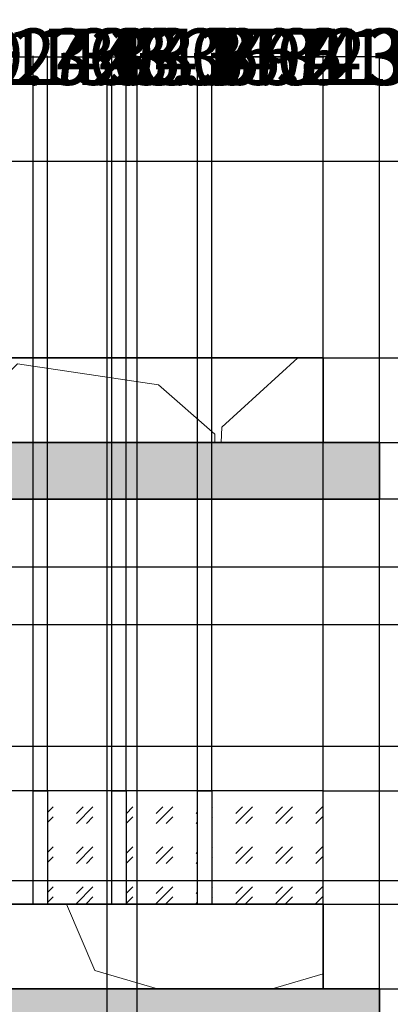
# Model space of a CAD drawing. Units: inches. Extents: x -73 to 458, y -161 to 332.
# Tile 5 of 6: x 259 to 338, y 123 to 332. Entities that reach past the tile are written whole.
import ezdxf

# ---------------------------------------------------------------- set-up
doc = ezdxf.new("R2010")
doc.units = ezdxf.units.IN
doc.header["$MEASUREMENT"] = 0
for name, color, linetype, lineweight in [('A-ANNO-DIMS', 2, 'Continuous', 18), ('A-ELEV', 7, 'Continuous', 35), ('A-ELEV-PATT', 8, 'Continuous', 13), ('A-GLAZ', 3, 'Continuous', 25), ('A-GLAZ-PATT', 8, 'Continuous', 13)]:
    doc.layers.add(name, color=color, linetype=linetype, lineweight=lineweight)
doc.styles.get("Standard").update_dxf_attribs({"font": 'arial.ttf'})
doc.dimstyles.get("Standard").update_dxf_attribs({"dimtxt": 12, "dimasz": 0.18, "dimexe": 0.18, "dimexo": 0.0625, "dimgap": 0.09, "dimtad": 0, "dimtih": 1, "dimtoh": 1, "dimdec": 0, "dimzin": 0, "dimdsep": 46, "dimlunit": 3, "dimtxsty": 'Standard', "dimcen": 0.09, "dimadec": 0, "dimazin": 0, "dimtfac": 1, "dimtdec": 0, "dimtofl": 0, "dimtmove": 0, "dimatfit": 3, "dimfxl": 1, "dimtolj": 1, "dimtzin": 0, "dimarcsym": 0})

# ---------------------------------------------------------------- blocks, each defined once
blk = doc.blocks.new('*D8')
at = {"layer": 'A-ANNO-DIMS', "color": 0, "lineweight": -2, "transparency": 16777216}
for p, q in [((204, 24.13), (204, 324.4)), ((204.18, 324.22), (257.28, 324.22)), ((335.82, 324.22), (282.72, 324.22)), ((336, 126.13), (336, 324.4))]:
    blk.add_line(p, q, dxfattribs=at)
at = {"layer": 'A-ANNO-DIMS', "color": 0, "transparency": 16777216}
for points in [[(204.18, 324.25), (204.18, 324.19), (204, 324.22)], [(335.82, 324.25), (335.82, 324.19), (336, 324.22)]]:
    blk.add_solid(points, dxfattribs=at)
at = {"layer": 'Defpoints', "color": 0, "transparency": 16777216}
for p in [(336, 324.22), (336, 126.07), (204, 24.07)]:
    blk.add_point(p, dxfattribs=at)
at = {"layer": 'A-ANNO-DIMS', "color": 0, "transparency": 16777216, "insert": (270, 324.22), "char_height": 12, "attachment_point": 5}
blk.add_mtext('\\A1;132', dxfattribs=at)
blk = doc.blocks.new('*D21')
at = {"layer": 'A-ANNO-DIMS', "color": 0, "lineweight": -2, "transparency": 16777216}
for p, q in [((336.06, 126.07), (408.51, 126.07)), ((408.33, 126.07), (408.33, 126.25)), ((408.33, 126.25), (408.51, 126.25)), ((408.33, 114.25), (408.33, 125.89)), ((336.06, 114.07), (408.51, 114.07))]:
    blk.add_line(p, q, dxfattribs=at)
at = {"layer": 'A-ANNO-DIMS', "color": 0, "transparency": 16777216}
for points in [[(408.3, 125.89), (408.36, 125.89), (408.33, 126.07)], [(408.3, 114.25), (408.36, 114.25), (408.33, 114.07)]]:
    blk.add_solid(points, dxfattribs=at)
at = {"layer": 'Defpoints', "color": 0, "transparency": 16777216}
for p in [(336, 126.07), (408.33, 126.07), (336, 114.07)]:
    blk.add_point(p, dxfattribs=at)
at = {"layer": 'A-ANNO-DIMS', "color": 0, "transparency": 16777216, "insert": (416.56, 126.25), "char_height": 12, "attachment_point": 5}
blk.add_mtext('\\A1;12', dxfattribs=at)
blk = doc.blocks.new('*D22')
at = {"layer": 'A-ANNO-DIMS', "color": 0, "lineweight": -2, "transparency": 16777216}
for p, q in [((336.06, 230.21), (408.51, 230.21)), ((408.33, 230.03), (408.33, 184.35)), ((408.33, 126.25), (408.33, 171.92)), ((336.06, 126.07), (408.51, 126.07))]:
    blk.add_line(p, q, dxfattribs=at)
at = {"layer": 'A-ANNO-DIMS', "color": 0, "transparency": 16777216}
for points in [[(408.3, 230.03), (408.36, 230.03), (408.33, 230.21)], [(408.3, 126.25), (408.36, 126.25), (408.33, 126.07)]]:
    blk.add_solid(points, dxfattribs=at)
at = {"layer": 'Defpoints', "color": 0, "transparency": 16777216}
for p in [(336, 230.21), (408.33, 230.21), (336, 126.07)]:
    blk.add_point(p, dxfattribs=at)
at = {"layer": 'A-ANNO-DIMS', "color": 0, "transparency": 16777216, "insert": (408.33, 178.14), "char_height": 12, "attachment_point": 5}
blk.add_mtext('\\A1;104.14', dxfattribs=at)
blk = doc.blocks.new('*D23')
at = {"layer": 'A-ANNO-DIMS', "color": 0, "lineweight": -2, "transparency": 16777216}
for p, q in [((336.06, 242.21), (408.51, 242.21)), ((408.33, 242.21), (408.33, 242.39)), ((408.33, 242.39), (408.51, 242.39)), ((408.33, 230.39), (408.33, 242.03)), ((336.06, 230.21), (408.51, 230.21))]:
    blk.add_line(p, q, dxfattribs=at)
at = {"layer": 'A-ANNO-DIMS', "color": 0, "transparency": 16777216}
for points in [[(408.3, 242.03), (408.36, 242.03), (408.33, 242.21)], [(408.3, 230.39), (408.36, 230.39), (408.33, 230.21)]]:
    blk.add_solid(points, dxfattribs=at)
at = {"layer": 'Defpoints', "color": 0, "transparency": 16777216}
for p in [(336, 242.21), (408.33, 242.21), (336, 230.21)]:
    blk.add_point(p, dxfattribs=at)
at = {"layer": 'A-ANNO-DIMS', "color": 0, "transparency": 16777216, "insert": (416.56, 242.39), "char_height": 12, "attachment_point": 5}
blk.add_mtext('\\A1;12', dxfattribs=at)
blk = doc.blocks.new('*D24')
at = {"layer": 'A-ANNO-DIMS', "color": 0, "lineweight": -2, "transparency": 16777216}
for p, q in [((324.06, 260.21), (408.51, 260.21)), ((408.33, 260.03), (408.33, 257.42)), ((408.33, 242.39), (408.33, 244.99)), ((324.06, 242.21), (408.51, 242.21))]:
    blk.add_line(p, q, dxfattribs=at)
at = {"layer": 'A-ANNO-DIMS', "color": 0, "transparency": 16777216}
for points in [[(408.3, 260.03), (408.36, 260.03), (408.33, 260.21)], [(408.3, 242.39), (408.36, 242.39), (408.33, 242.21)]]:
    blk.add_solid(points, dxfattribs=at)
at = {"layer": 'Defpoints', "color": 0, "transparency": 16777216}
for p in [(324, 260.21), (408.33, 260.21), (324, 242.21)]:
    blk.add_point(p, dxfattribs=at)
at = {"layer": 'A-ANNO-DIMS', "color": 0, "transparency": 16777216, "insert": (408.33, 251.21), "char_height": 12, "attachment_point": 5}
blk.add_mtext('\\A1;18', dxfattribs=at)
blk = doc.blocks.new('*D25')
at = {"layer": 'A-ANNO-DIMS', "color": 0, "lineweight": -2, "transparency": 16777216}
for p, q in [((168.06, 302.02), (408.51, 302.02)), ((408.33, 301.84), (408.33, 287.33)), ((408.33, 260.39), (408.33, 274.9)), ((168.06, 260.21), (408.51, 260.21))]:
    blk.add_line(p, q, dxfattribs=at)
at = {"layer": 'A-ANNO-DIMS', "color": 0, "transparency": 16777216}
for points in [[(408.3, 301.84), (408.36, 301.84), (408.33, 302.02)], [(408.3, 260.39), (408.36, 260.39), (408.33, 260.21)]]:
    blk.add_solid(points, dxfattribs=at)
at = {"layer": 'Defpoints', "color": 0, "transparency": 16777216}
for p in [(168, 302.02), (408.33, 302.02), (168, 260.21)]:
    blk.add_point(p, dxfattribs=at)
at = {"layer": 'A-ANNO-DIMS', "color": 0, "transparency": 16777216, "insert": (408.33, 281.11), "char_height": 12, "attachment_point": 5}
blk.add_mtext('\\A1;41.814', dxfattribs=at)
blk = doc.blocks.new('*D42')
at = {"layer": 'A-ANNO-DIMS', "color": 0, "lineweight": -2, "transparency": 16777216}
for p, q in [((144.06, 149.14), (408.51, 149.14)), ((408.33, 148.96), (408.33, 140.32)), ((408.33, 119.24), (408.33, 127.88)), ((144.06, 119.06), (408.51, 119.06))]:
    blk.add_line(p, q, dxfattribs=at)
at = {"layer": 'A-ANNO-DIMS', "color": 0, "transparency": 16777216}
for points in [[(408.3, 148.96), (408.36, 148.96), (408.33, 149.14)], [(408.3, 119.24), (408.36, 119.24), (408.33, 119.06)]]:
    blk.add_solid(points, dxfattribs=at)
at = {"layer": 'Defpoints', "color": 0, "transparency": 16777216}
for p in [(144, 149.14), (408.33, 149.14), (144, 119.06)]:
    blk.add_point(p, dxfattribs=at)
at = {"layer": 'A-ANNO-DIMS', "color": 0, "transparency": 16777216, "insert": (408.33, 134.1), "char_height": 12, "attachment_point": 5}
blk.add_mtext('\\A1;30.08', dxfattribs=at)
blk = doc.blocks.new('*D43')
at = {"layer": 'A-ANNO-DIMS', "color": 0, "lineweight": -2, "transparency": 16777216}
for p, q in [((144.06, 177.7), (408.51, 177.7)), ((408.33, 177.52), (408.33, 169.64)), ((408.33, 149.32), (408.33, 157.2)), ((144.06, 149.14), (408.51, 149.14))]:
    blk.add_line(p, q, dxfattribs=at)
at = {"layer": 'A-ANNO-DIMS', "color": 0, "transparency": 16777216}
for points in [[(408.3, 177.52), (408.36, 177.52), (408.33, 177.7)], [(408.3, 149.32), (408.36, 149.32), (408.33, 149.14)]]:
    blk.add_solid(points, dxfattribs=at)
at = {"layer": 'Defpoints', "color": 0, "transparency": 16777216}
for p in [(144, 177.7), (408.33, 177.7), (144, 149.14)]:
    blk.add_point(p, dxfattribs=at)
at = {"layer": 'A-ANNO-DIMS', "color": 0, "transparency": 16777216, "insert": (408.33, 163.42), "char_height": 12, "attachment_point": 5}
blk.add_mtext('\\A1;28.57', dxfattribs=at)
blk = doc.blocks.new('*D44')
at = {"layer": 'A-ANNO-DIMS', "color": 0, "lineweight": -2, "transparency": 16777216}
for p, q in [((144.06, 203.54), (408.51, 203.54)), ((408.33, 203.36), (408.33, 196.84)), ((408.33, 177.88), (408.33, 184.4)), ((144.06, 177.7), (408.51, 177.7))]:
    blk.add_line(p, q, dxfattribs=at)
at = {"layer": 'A-ANNO-DIMS', "color": 0, "transparency": 16777216}
for points in [[(408.3, 203.36), (408.36, 203.36), (408.33, 203.54)], [(408.3, 177.88), (408.36, 177.88), (408.33, 177.7)]]:
    blk.add_solid(points, dxfattribs=at)
at = {"layer": 'Defpoints', "color": 0, "transparency": 16777216}
for p in [(144, 203.54), (408.33, 203.54), (144, 177.7)]:
    blk.add_point(p, dxfattribs=at)
at = {"layer": 'A-ANNO-DIMS', "color": 0, "transparency": 16777216, "insert": (408.33, 190.62), "char_height": 12, "attachment_point": 5}
blk.add_mtext('\\A1;25.83', dxfattribs=at)
blk = doc.blocks.new('*D45')
at = {"layer": 'A-ANNO-DIMS', "color": 0, "lineweight": -2, "transparency": 16777216}
for p, q in [((144.06, 215.8), (408.51, 215.8)), ((408.33, 215.8), (408.33, 215.98)), ((408.33, 215.98), (408.51, 215.98)), ((408.33, 203.72), (408.33, 215.62)), ((144.06, 203.54), (408.51, 203.54))]:
    blk.add_line(p, q, dxfattribs=at)
at = {"layer": 'A-ANNO-DIMS', "color": 0, "transparency": 16777216}
for points in [[(408.3, 215.62), (408.36, 215.62), (408.33, 215.8)], [(408.3, 203.72), (408.36, 203.72), (408.33, 203.54)]]:
    blk.add_solid(points, dxfattribs=at)
at = {"layer": 'Defpoints', "color": 0, "transparency": 16777216}
for p in [(144, 215.8), (408.33, 215.8), (144, 203.54)]:
    blk.add_point(p, dxfattribs=at)
at = {"layer": 'A-ANNO-DIMS', "color": 0, "transparency": 16777216, "insert": (432.98, 215.98), "char_height": 12, "attachment_point": 5}
blk.add_mtext('\\A1;12.265', dxfattribs=at)
blk = doc.blocks.new('*D46')
at = {"layer": 'A-ANNO-DIMS', "color": 0, "lineweight": -2, "transparency": 16777216}
for p, q in [((156.06, 230.21), (408.51, 230.21)), ((408.33, 230.03), (408.33, 229.22)), ((144.06, 215.8), (408.51, 215.8)), ((408.33, 215.98), (408.33, 216.79))]:
    blk.add_line(p, q, dxfattribs=at)
at = {"layer": 'A-ANNO-DIMS', "color": 0, "transparency": 16777216}
for points in [[(408.3, 230.03), (408.36, 230.03), (408.33, 230.21)], [(408.3, 215.98), (408.36, 215.98), (408.33, 215.8)]]:
    blk.add_solid(points, dxfattribs=at)
at = {"layer": 'Defpoints', "color": 0, "transparency": 16777216}
for p in [(156, 230.21), (408.33, 230.21), (144, 215.8)]:
    blk.add_point(p, dxfattribs=at)
at = {"layer": 'A-ANNO-DIMS', "color": 0, "transparency": 16777216, "insert": (408.33, 223), "char_height": 12, "attachment_point": 5}
blk.add_mtext('\\A1;14.406', dxfattribs=at)
blk = doc.blocks.new('*D54')
at = {"layer": 'A-ANNO-DIMS', "color": 0, "lineweight": -2, "transparency": 16777216}
for p, q in [((249, 168.25), (249, 324.4)), ((249.18, 324.22), (262.15, 324.22)), ((262.33, 168.25), (262.33, 324.4)), ((262.33, 324.22), (262.51, 324.22))]:
    blk.add_line(p, q, dxfattribs=at)
at = {"layer": 'A-ANNO-DIMS', "color": 0, "transparency": 16777216}
for points in [[(249.18, 324.25), (249.18, 324.19), (249, 324.22)], [(262.15, 324.25), (262.15, 324.19), (262.33, 324.22)]]:
    blk.add_solid(points, dxfattribs=at)
at = {"layer": 'Defpoints', "color": 0, "transparency": 16777216}
for p in [(262.33, 324.22), (249, 168.19), (262.33, 168.19)]:
    blk.add_point(p, dxfattribs=at)
at = {"layer": 'A-ANNO-DIMS', "color": 0, "transparency": 16777216, "insert": (282.28, 324.22), "char_height": 12, "attachment_point": 5}
blk.add_mtext('\\A1;13.33', dxfattribs=at)
blk = doc.blocks.new('*D55')
at = {"layer": 'A-ANNO-DIMS', "color": 0, "lineweight": -2, "transparency": 16777216}
for p, q in [((262.33, 168.25), (262.33, 324.4)), ((262.51, 324.22), (265.19, 324.22)), ((265.37, 168.25), (265.37, 324.4)), ((265.37, 324.22), (265.55, 324.22))]:
    blk.add_line(p, q, dxfattribs=at)
at = {"layer": 'A-ANNO-DIMS', "color": 0, "transparency": 16777216}
for points in [[(262.51, 324.25), (262.51, 324.19), (262.33, 324.22)], [(265.19, 324.25), (265.19, 324.19), (265.37, 324.22)]]:
    blk.add_solid(points, dxfattribs=at)
at = {"layer": 'Defpoints', "color": 0, "transparency": 16777216}
for p in [(265.37, 324.22), (262.33, 168.19), (265.37, 168.19)]:
    blk.add_point(p, dxfattribs=at)
at = {"layer": 'A-ANNO-DIMS', "color": 0, "transparency": 16777216, "insert": (285.88, 324.22), "char_height": 12, "attachment_point": 5}
blk.add_mtext('\\A1;3.043', dxfattribs=at)
blk = doc.blocks.new('*D56')
at = {"layer": 'A-ANNO-DIMS', "color": 0, "lineweight": -2, "transparency": 16777216}
for p, q in [((265.37, 168.25), (265.37, 324.4)), ((265.55, 324.22), (278.88, 324.22)), ((279.06, 168.25), (279.06, 324.4)), ((279.06, 324.22), (279.24, 324.22))]:
    blk.add_line(p, q, dxfattribs=at)
at = {"layer": 'A-ANNO-DIMS', "color": 0, "transparency": 16777216}
for points in [[(265.55, 324.25), (265.55, 324.19), (265.37, 324.22)], [(278.88, 324.25), (278.88, 324.19), (279.06, 324.22)]]:
    blk.add_solid(points, dxfattribs=at)
at = {"layer": 'Defpoints', "color": 0, "transparency": 16777216}
for p in [(279.06, 324.22), (265.37, 168.19), (279.06, 168.19)]:
    blk.add_point(p, dxfattribs=at)
at = {"layer": 'A-ANNO-DIMS', "color": 0, "transparency": 16777216, "insert": (303.65, 324.22), "char_height": 12, "attachment_point": 5}
blk.add_mtext('\\A1;13.694', dxfattribs=at)
blk = doc.blocks.new('*D57')
at = {"layer": 'A-ANNO-DIMS', "color": 0, "lineweight": -2, "transparency": 16777216}
for p, q in [((279.06, 168.25), (279.06, 324.4)), ((279.24, 324.22), (281.93, 324.22)), ((282.11, 168.25), (282.11, 324.4)), ((282.11, 324.22), (282.29, 324.22))]:
    blk.add_line(p, q, dxfattribs=at)
at = {"layer": 'A-ANNO-DIMS', "color": 0, "transparency": 16777216}
for points in [[(279.24, 324.25), (279.24, 324.19), (279.06, 324.22)], [(281.93, 324.25), (281.93, 324.19), (282.11, 324.22)]]:
    blk.add_solid(points, dxfattribs=at)
at = {"layer": 'Defpoints', "color": 0, "transparency": 16777216}
for p in [(282.11, 324.22), (279.06, 168.19), (282.11, 168.19)]:
    blk.add_point(p, dxfattribs=at)
at = {"layer": 'A-ANNO-DIMS', "color": 0, "transparency": 16777216, "insert": (302.62, 324.22), "char_height": 12, "attachment_point": 5}
blk.add_mtext('\\A1;3.043', dxfattribs=at)
blk = doc.blocks.new('*D58')
at = {"layer": 'A-ANNO-DIMS', "color": 0, "lineweight": -2, "transparency": 16777216}
for p, q in [((282.11, 168.25), (282.11, 324.4)), ((282.29, 324.22), (297.14, 324.22)), ((297.32, 168.25), (297.32, 324.4)), ((297.32, 324.22), (297.5, 324.22))]:
    blk.add_line(p, q, dxfattribs=at)
at = {"layer": 'A-ANNO-DIMS', "color": 0, "transparency": 16777216}
for points in [[(282.29, 324.25), (282.29, 324.19), (282.11, 324.22)], [(297.14, 324.25), (297.14, 324.19), (297.32, 324.22)]]:
    blk.add_solid(points, dxfattribs=at)
at = {"layer": 'Defpoints', "color": 0, "transparency": 16777216}
for p in [(297.32, 324.22), (282.11, 168.19), (297.32, 168.19)]:
    blk.add_point(p, dxfattribs=at)
at = {"layer": 'A-ANNO-DIMS', "color": 0, "transparency": 16777216, "insert": (321.93, 324.22), "char_height": 12, "attachment_point": 5}
blk.add_mtext('\\A1;15.216', dxfattribs=at)
blk = doc.blocks.new('*D59')
at = {"layer": 'A-ANNO-DIMS', "color": 0, "lineweight": -2, "transparency": 16777216}
for p, q in [((297.32, 168.25), (297.32, 324.4)), ((297.5, 324.22), (300.19, 324.22)), ((300.37, 168.25), (300.37, 324.4)), ((300.37, 324.22), (300.55, 324.22))]:
    blk.add_line(p, q, dxfattribs=at)
at = {"layer": 'A-ANNO-DIMS', "color": 0, "transparency": 16777216}
for points in [[(297.5, 324.25), (297.5, 324.19), (297.32, 324.22)], [(300.19, 324.25), (300.19, 324.19), (300.37, 324.22)]]:
    blk.add_solid(points, dxfattribs=at)
at = {"layer": 'Defpoints', "color": 0, "transparency": 16777216}
for p in [(300.37, 324.22), (297.32, 168.19), (300.37, 168.19)]:
    blk.add_point(p, dxfattribs=at)
at = {"layer": 'A-ANNO-DIMS', "color": 0, "transparency": 16777216, "insert": (320.88, 324.22), "char_height": 12, "attachment_point": 5}
blk.add_mtext('\\A1;3.043', dxfattribs=at)
blk = doc.blocks.new('*D60')
at = {"layer": 'A-ANNO-DIMS', "color": 0, "lineweight": -2, "transparency": 16777216}
for p, q in [((300.37, 168.25), (300.37, 324.4)), ((300.55, 324.22), (323.82, 324.22)), ((324, 168.25), (324, 324.4)), ((324, 324.22), (324.18, 324.22))]:
    blk.add_line(p, q, dxfattribs=at)
at = {"layer": 'A-ANNO-DIMS', "color": 0, "transparency": 16777216}
for points in [[(300.55, 324.25), (300.55, 324.19), (300.37, 324.22)], [(323.82, 324.25), (323.82, 324.19), (324, 324.22)]]:
    blk.add_solid(points, dxfattribs=at)
at = {"layer": 'Defpoints', "color": 0, "transparency": 16777216}
for p in [(324, 324.22), (300.37, 168.19), (324, 168.19)]:
    blk.add_point(p, dxfattribs=at)
at = {"layer": 'A-ANNO-DIMS', "color": 0, "transparency": 16777216, "insert": (344.62, 324.22), "char_height": 12, "attachment_point": 5}
blk.add_mtext('\\A1;23.63', dxfattribs=at)
blk = doc.blocks.new('*D69')
at = {"layer": 'A-ANNO-DIMS', "color": 0, "lineweight": -2, "transparency": 16777216}
for p, q in [((324.06, 168.19), (408.51, 168.19)), ((408.33, 168.01), (408.33, 162.35)), ((408.33, 144.25), (408.33, 149.91)), ((324.06, 144.07), (408.51, 144.07))]:
    blk.add_line(p, q, dxfattribs=at)
at = {"layer": 'A-ANNO-DIMS', "color": 0, "transparency": 16777216}
for points in [[(408.3, 168.01), (408.36, 168.01), (408.33, 168.19)], [(408.3, 144.25), (408.36, 144.25), (408.33, 144.07)]]:
    blk.add_solid(points, dxfattribs=at)
at = {"layer": 'Defpoints', "color": 0, "transparency": 16777216}
for p in [(324, 168.19), (408.33, 168.19), (324, 144.07)]:
    blk.add_point(p, dxfattribs=at)
at = {"layer": 'A-ANNO-DIMS', "color": 0, "transparency": 16777216, "insert": (408.33, 156.13), "char_height": 12, "attachment_point": 5}
blk.add_mtext('\\A1;24.125', dxfattribs=at)
blk = doc.blocks.new('*D72')
at = {"layer": 'A-ANNO-DIMS', "color": 0, "lineweight": -2, "transparency": 16777216}
for p, q in [((202.35, -5.87), (202.35, 324.4)), ((202.53, 324.22), (241.93, 324.22)), ((242.11, -5.87), (242.11, 324.4)), ((242.11, 324.22), (242.29, 324.22))]:
    blk.add_line(p, q, dxfattribs=at)
at = {"layer": 'A-ANNO-DIMS', "color": 0, "transparency": 16777216}
for points in [[(202.53, 324.25), (202.53, 324.19), (202.35, 324.22)], [(241.93, 324.25), (241.93, 324.19), (242.11, 324.22)]]:
    blk.add_solid(points, dxfattribs=at)
at = {"layer": 'Defpoints', "color": 0, "transparency": 16777216}
for p in [(242.11, 324.22), (202.35, -5.93), (242.11, -5.93)]:
    blk.add_point(p, dxfattribs=at)
at = {"layer": 'A-ANNO-DIMS', "color": 0, "transparency": 16777216, "insert": (262.62, 324.22), "char_height": 12, "attachment_point": 5}
blk.add_mtext('\\A1;39.76', dxfattribs=at)
blk = doc.blocks.new('*D73')
at = {"layer": 'A-ANNO-DIMS', "color": 0, "lineweight": -2, "transparency": 16777216}
for p, q in [((242.11, -5.87), (242.11, 324.4)), ((242.29, 324.22), (244.17, 324.22)), ((244.35, -5.87), (244.35, 324.4)), ((244.35, 324.22), (244.53, 324.22))]:
    blk.add_line(p, q, dxfattribs=at)
at = {"layer": 'A-ANNO-DIMS', "color": 0, "transparency": 16777216}
for points in [[(242.29, 324.25), (242.29, 324.19), (242.11, 324.22)], [(244.17, 324.25), (244.17, 324.19), (244.35, 324.22)]]:
    blk.add_solid(points, dxfattribs=at)
at = {"layer": 'Defpoints', "color": 0, "transparency": 16777216}
for p in [(244.35, 324.22), (242.11, -5.93), (244.35, -5.93)]:
    blk.add_point(p, dxfattribs=at)
at = {"layer": 'A-ANNO-DIMS', "color": 0, "transparency": 16777216, "insert": (264.95, 324.22), "char_height": 12, "attachment_point": 5}
blk.add_mtext('\\A1;2.244', dxfattribs=at)
blk = doc.blocks.new('*D74')
at = {"layer": 'A-ANNO-DIMS', "color": 0, "lineweight": -2, "transparency": 16777216}
for p, q in [((244.35, -5.87), (244.35, 324.4)), ((244.53, 324.22), (277.93, 324.22)), ((278.11, -5.87), (278.11, 324.4)), ((278.11, 324.22), (278.29, 324.22))]:
    blk.add_line(p, q, dxfattribs=at)
at = {"layer": 'A-ANNO-DIMS', "color": 0, "transparency": 16777216}
for points in [[(244.53, 324.25), (244.53, 324.19), (244.35, 324.22)], [(277.93, 324.25), (277.93, 324.19), (278.11, 324.22)]]:
    blk.add_solid(points, dxfattribs=at)
at = {"layer": 'Defpoints', "color": 0, "transparency": 16777216}
for p in [(278.11, 324.22), (244.35, -5.93), (278.11, -5.93)]:
    blk.add_point(p, dxfattribs=at)
at = {"layer": 'A-ANNO-DIMS', "color": 0, "transparency": 16777216, "insert": (303.28, 324.22), "char_height": 12, "attachment_point": 5}
blk.add_mtext('\\A1;33.756', dxfattribs=at)
blk = doc.blocks.new('*D75')
at = {"layer": 'A-ANNO-DIMS', "color": 0, "lineweight": -2, "transparency": 16777216}
for p, q in [((278.11, -5.87), (278.11, 324.4)), ((278.29, 324.22), (284.3, 324.22)), ((284.48, -5.87), (284.48, 324.4)), ((284.48, 324.22), (284.66, 324.22))]:
    blk.add_line(p, q, dxfattribs=at)
at = {"layer": 'A-ANNO-DIMS', "color": 0, "transparency": 16777216}
for points in [[(278.29, 324.25), (278.29, 324.19), (278.11, 324.22)], [(284.3, 324.25), (284.3, 324.19), (284.48, 324.22)]]:
    blk.add_solid(points, dxfattribs=at)
at = {"layer": 'Defpoints', "color": 0, "transparency": 16777216}
for p in [(284.48, 324.22), (278.11, -5.93), (284.48, -5.93)]:
    blk.add_point(p, dxfattribs=at)
at = {"layer": 'A-ANNO-DIMS', "color": 0, "transparency": 16777216, "insert": (305.03, 324.22), "char_height": 12, "attachment_point": 5}
blk.add_mtext('\\A1;6.377', dxfattribs=at)

msp = doc.modelspace()

# ---------------------------------------------------------------- hatches: boundary and pattern name
at = {"layer": 'A-ELEV-PATT'}
h = msp.add_hatch(color=256, dxfattribs=at)
h.dxf.hatch_style = 1
h.paths.add_polyline_path([(167.9979, 302.0202), (155.9979, 302.0202), (95.9979, 302.0202), (23.9979, 302.0202), (23.9979, -113.9335), (33.9979, -113.9335), (33.9979, 292.0202), (95.9979, 292.0202), (157.9979, 292.0202), (157.9979, 260.2059), (167.9979, 260.2059), (167.9979, 290.0202)])
h.paths.add_polyline_path([(335.9979, 242.2059), (323.9979, 242.2059), (95.9979, 242.2059), (95.9979, 234.0665), (95.9979, 230.2059), (323.9979, 230.2059), (335.9979, 230.2059)])
h.paths.add_polyline_path([(335.9979, 126.0665), (323.9979, 126.0665), (173.9979, 126.0665), (173.9979, 114.0665), (323.9979, 114.0665), (335.9979, 114.0665)])
h.paths.add_polyline_path([(335.9979, 6.0665), (323.9979, 6.0665), (95.9979, 6.0665), (95.9979, -5.9335), (323.9979, -5.9335), (335.9979, -5.9335)])
h = msp.add_hatch(dxfattribs=at)
h.set_pattern_fill('GRAVEL', color=256, scale=150)
h.paths.add_polyline_path([(95.9979, 234.0665), (95.9979, 260.2059), (155.9979, 260.2059), (155.9979, 290.0202), (95.9979, 290.0202), (55.9979, 290.0202), (55.9979, -113.9335), (95.9979, -113.9335), (95.9979, 24.0665), (95.9979, 54.0267)])
h.paths.add_polyline_path([(323.9979, 144.0665), (248.9979, 144.0665), (173.9979, 144.0665), (173.9979, 126.0665), (323.9979, 126.0665)])
h.paths.add_polyline_path([(323.9979, 24.0665), (248.9979, 24.0665), (155.9979, 24.0665), (155.9979, 6.0665), (323.9979, 6.0665)])
h.paths.add_polyline_path([(323.9979, 260.2059), (95.9979, 260.2059), (95.9979, 242.2059), (323.9979, 242.2059)])
h.paths.add_polyline_path([(155.9979, 24.0665), (95.9979, 24.0665), (95.9979, 6.0665), (155.9979, 6.0665)], flags=17)

# ---------------------------------------------------------------- linework, layer by layer
at = {"layer": 'A-ELEV'}
for p, q in [((323.9979, 260.2059), (95.9979, 260.2059)), ((323.9979, 260.2059), (323.9979, 242.2059)), ((323.9979, 242.2059), (95.9979, 242.2059)), ((323.9979, 230.2059), (95.9979, 230.2059)), ((323.9979, 144.0665), (173.9979, 144.0665)), ((323.9979, 144.0665), (323.9979, 126.0665)), ((323.9979, 126.0665), (173.9979, 126.0665))]:
    msp.add_line(p, q, dxfattribs=at)
for points in [[(323.9979, 242.2059), (335.9979, 242.2059), (335.9979, 230.2059), (323.9979, 230.2059)], [(323.9979, 126.0665), (335.9979, 126.0665), (335.9979, 114.0665), (323.9979, 114.0665)]]:
    msp.add_lwpolyline(points, dxfattribs=at)
at = {"layer": 'A-GLAZ'}
for points in [[(248.9979, 144.0665), (323.9979, 144.0665), (323.9979, 168.1912), (248.9979, 168.1912)], [(262.3267, 168.1912), (265.3698, 168.1912), (265.3698, 144.0665), (262.3267, 144.0665)], [(279.0639, 168.1912), (282.107, 168.1912), (282.107, 144.0665), (279.0639, 144.0665)], [(297.3226, 168.1912), (300.3657, 168.1912), (300.3657, 144.0665), (297.3226, 144.0665)]]:
    msp.add_lwpolyline(points, close=True, dxfattribs=at)
at = {"layer": 'A-GLAZ-PATT'}
for p, q in [((265.3698, 163.5465), (266.5793, 164.7559)), ((271.529, 161.2203), (275.0645, 164.7559)), ((271.529, 163.3417), (272.9432, 164.7559)), ((282.107, 163.3131), (283.5498, 164.7559)), ((288.4996, 161.2203), (292.0351, 164.7559)), ((288.4996, 163.3417), (289.9138, 164.7559)), ((296.9848, 163.3417), (297.3226, 163.6794)), ((300.3657, 164.6012), (300.5204, 164.7559)), ((305.4701, 161.2203), (309.0057, 164.7559)), ((305.4701, 163.3417), (306.8843, 164.7559)), ((313.9554, 161.2203), (317.4909, 164.7559)), ((313.9554, 163.3417), (315.3696, 164.7559)), ((322.4407, 163.3417), (323.8549, 164.7559)), ((265.3698, 161.4251), (266.5793, 162.6346)), ((273.6503, 161.2203), (275.0645, 162.6346)), ((282.1356, 161.2203), (283.5498, 162.6346)), ((290.6209, 161.2203), (292.0351, 162.6346)), ((296.9848, 161.2203), (297.3226, 161.5581)), ((300.3657, 162.4799), (300.5204, 162.6346)), ((307.5914, 161.2203), (309.0057, 162.6346)), ((316.0767, 161.2203), (317.4909, 162.6346)), ((322.4407, 161.2203), (323.9979, 162.7775)), ((265.3698, 155.0612), (266.5793, 156.2706)), ((271.529, 152.7351), (275.0645, 156.2706)), ((271.529, 154.8564), (272.9432, 156.2706)), ((282.107, 154.8278), (283.5498, 156.2706)), ((288.4996, 152.7351), (292.0351, 156.2706)), ((288.4996, 154.8564), (289.9138, 156.2706)), ((296.9848, 154.8564), (297.3226, 155.1941)), ((300.3657, 156.116), (300.5204, 156.2706)), ((305.4701, 152.7351), (309.0057, 156.2706)), ((305.4701, 154.8564), (306.8843, 156.2706)), ((313.9554, 152.7351), (317.4909, 156.2706)), ((313.9554, 154.8564), (315.3696, 156.2706)), ((322.4407, 154.8564), (323.8549, 156.2706)), ((265.3698, 152.9398), (266.5793, 154.1493)), ((273.6503, 152.7351), (275.0645, 154.1493)), ((282.1356, 152.7351), (283.5498, 154.1493)), ((290.6209, 152.7351), (292.0351, 154.1493)), ((296.9848, 152.7351), (297.3226, 153.0728)), ((300.3657, 153.9946), (300.5204, 154.1493)), ((307.5914, 152.7351), (309.0057, 154.1493)), ((316.0767, 152.7351), (317.4909, 154.1493)), ((322.4407, 152.7351), (323.9979, 154.2922)), ((265.3698, 146.5759), (266.5793, 147.7853)), ((271.529, 144.2498), (275.0645, 147.7853)), ((271.529, 146.3711), (272.9432, 147.7853)), ((282.107, 146.3425), (283.5498, 147.7853)), ((288.4996, 144.2498), (292.0351, 147.7853)), ((288.4996, 146.3711), (289.9138, 147.7853)), ((296.9848, 146.3711), (297.3226, 146.7089)), ((300.3657, 147.6307), (300.5204, 147.7853)), ((305.4701, 144.2498), (309.0057, 147.7853)), ((305.4701, 146.3711), (306.8843, 147.7853)), ((313.9554, 144.2498), (317.4909, 147.7853)), ((313.9554, 146.3711), (315.3696, 147.7853)), ((322.4407, 146.3711), (323.8549, 147.7853)), ((265.3698, 144.4546), (266.5793, 145.664)), ((273.6503, 144.2498), (275.0645, 145.664)), ((282.1356, 144.2498), (283.5498, 145.664)), ((290.6209, 144.2498), (292.0351, 145.664)), ((296.9848, 144.2498), (297.3226, 144.5875)), ((300.3657, 145.5094), (300.5204, 145.664)), ((307.5914, 144.2498), (309.0057, 145.664)), ((316.0767, 144.2498), (317.4909, 145.664)), ((322.4407, 144.2498), (323.9979, 145.807))]:
    msp.add_line(p, q, dxfattribs=at)

# ---------------------------------------------------------------- dimensions: what is measured, and where the dimension line sits
at = {"layer": 'A-ANNO-DIMS'}
for base, p1, p2, override, picture, middle in [((242.1074, 324.2202), (202.3513, -5.9335), (242.1074, -5.9335), {"dimdec": 2, "dimlfac": 1, "dimrnd": 0, "dimzin": 0, "dimdsep": 46, "dimlunit": 2}, '*D72', (262.6161, 324.2202)), ((335.9979, 324.2202), (203.9979, 24.0665), (335.9979, 126.0665), {"dimdec": 0, "dimlfac": 1, "dimrnd": 0, "dimzin": 0, "dimdsep": 46, "dimlunit": 2}, '*D8', (269.9979, 324.2202)), ((244.3513, 324.2202), (242.1074, -5.9335), (244.3513, -5.9335), {"dimdec": 3, "dimlfac": 1, "dimrnd": 0, "dimzin": 0, "dimdsep": 46, "dimlunit": 2}, '*D73', (264.946, 324.2202)), ((278.1074, 324.2202), (244.3513, -5.9335), (278.1074, -5.9335), {"dimdec": 3, "dimlfac": 1, "dimrnd": 0, "dimzin": 0, "dimdsep": 46, "dimlunit": 2}, '*D74', (303.2778, 324.2202)), ((262.3267, 324.2202), (248.9979, 168.1912), (262.3267, 168.1912), {"dimdec": 2, "dimlfac": 1, "dimrnd": 0, "dimzin": 0, "dimdsep": 46, "dimlunit": 2}, '*D54', (282.2788, 324.2202)), ((265.3698, 324.2202), (262.3267, 168.1912), (265.3698, 168.1912), {"dimdec": 3, "dimlfac": 1, "dimrnd": 0, "dimzin": 0, "dimdsep": 46, "dimlunit": 2}, '*D55', (285.8827, 324.2202)), ((279.0639, 324.2202), (265.3698, 168.1912), (279.0639, 168.1912), {"dimdec": 3, "dimlfac": 1, "dimrnd": 0, "dimzin": 0, "dimdsep": 46, "dimlunit": 2}, '*D56', (303.6531, 324.2202)), ((284.4845, 324.2202), (278.1074, -5.9335), (284.4845, -5.9335), {"dimdec": 3, "dimlfac": 1, "dimrnd": 0, "dimzin": 0, "dimdsep": 46, "dimlunit": 2}, '*D75', (305.0342, 324.2202)), ((282.107, 324.2202), (279.0639, 168.1912), (282.107, 168.1912), {"dimdec": 3, "dimlfac": 1, "dimrnd": 0, "dimzin": 0, "dimdsep": 46, "dimlunit": 2}, '*D57', (302.6198, 324.2202)), ((297.3226, 324.2202), (282.107, 168.1912), (297.3226, 168.1912), {"dimdec": 3, "dimlfac": 1, "dimrnd": 0, "dimzin": 0, "dimdsep": 46, "dimlunit": 2}, '*D58', (321.9323, 324.2202)), ((300.3657, 324.2202), (297.3226, 168.1912), (300.3657, 168.1912), {"dimdec": 3, "dimlfac": 1, "dimrnd": 0, "dimzin": 0, "dimdsep": 46, "dimlunit": 2}, '*D59', (320.8786, 324.2202)), ((323.9979, 324.2202), (300.3657, 168.1912), (323.9979, 168.1912), {"dimdec": 2, "dimlfac": 1, "dimrnd": 0, "dimzin": 0, "dimdsep": 46, "dimlunit": 2}, '*D60', (344.6171, 324.2202))]:
    dim = msp.add_linear_dim(base=base, p1=p1, p2=p2, dimstyle='Standard', override=override, dxfattribs=at)
    dim.commit()
    dim.dimension.update_dxf_attribs({"geometry": picture, "text_midpoint": middle})
for base, p1, p2, override, picture, middle in [((408.326, 302.0202), (167.9979, 260.2059), (167.9979, 302.0202), {"dimdec": 3, "dimlfac": 1, "dimrnd": 0, "dimzin": 0, "dimdsep": 46, "dimlunit": 2}, '*D25', (408.326, 281.1131)), ((408.326, 260.2059), (323.9979, 242.2059), (323.9979, 260.2059), {"dimdec": 0, "dimlfac": 1, "dimrnd": 0, "dimzin": 0, "dimdsep": 46, "dimlunit": 2}, '*D24', (408.326, 251.2059)), ((408.326, 242.2059), (335.9979, 230.2059), (335.9979, 242.2059), {"dimdec": 0, "dimlfac": 1, "dimrnd": 0, "dimzin": 0, "dimdsep": 46, "dimlunit": 2}, '*D23', (416.5646, 242.3859)), ((408.326, 230.2059), (143.9979, 215.8003), (155.9979, 230.2059), {"dimdec": 3, "dimlfac": 1, "dimrnd": 0, "dimzin": 0, "dimdsep": 46, "dimlunit": 2}, '*D46', (408.326, 223.0031)), ((408.326, 230.2059), (335.9979, 126.0665), (335.9979, 230.2059), {"dimdec": 2, "dimlfac": 1, "dimrnd": 0, "dimzin": 0, "dimdsep": 46, "dimlunit": 2}, '*D22', (408.326, 178.1362)), ((408.326, 215.8003), (143.9979, 203.5354), (143.9979, 215.8003), {"dimdec": 3, "dimlfac": 1, "dimrnd": 0, "dimzin": 0, "dimdsep": 46, "dimlunit": 2}, '*D45', (432.9848, 215.9803)), ((408.326, 203.5354), (143.9979, 177.7045), (143.9979, 203.5354), {"dimdec": 2, "dimlfac": 1, "dimrnd": 0, "dimzin": 0, "dimdsep": 46, "dimlunit": 2}, '*D44', (408.326, 190.6199)), ((408.326, 177.7045), (143.9979, 149.136), (143.9979, 177.7045), {"dimdec": 2, "dimlfac": 1, "dimrnd": 0, "dimzin": 0, "dimdsep": 46, "dimlunit": 2}, '*D43', (408.326, 163.4203)), ((408.326, 168.1912), (323.9979, 144.0665), (323.9979, 168.1912), {"dimdec": 3, "dimlfac": 1, "dimrnd": 0, "dimzin": 0, "dimdsep": 46, "dimlunit": 2}, '*D69', (408.326, 156.1288)), ((408.326, 149.136), (143.9979, 119.0564), (143.9979, 149.136), {"dimdec": 2, "dimlfac": 1, "dimrnd": 0, "dimzin": 0, "dimdsep": 46, "dimlunit": 2}, '*D42', (408.326, 134.0962)), ((408.326, 126.0665), (335.9979, 114.0665), (335.9979, 126.0665), {"dimdec": 0, "dimlfac": 1, "dimrnd": 0, "dimzin": 0, "dimdsep": 46, "dimlunit": 2}, '*D21', (416.5646, 126.2465))]:
    dim = msp.add_linear_dim(base=base, p1=p1, p2=p2, angle=90, dimstyle='Standard', override=override, dxfattribs=at)
    dim.commit()
    dim.dimension.update_dxf_attribs({"geometry": picture, "text_midpoint": middle})

doc.saveas('drawing.dxf')
